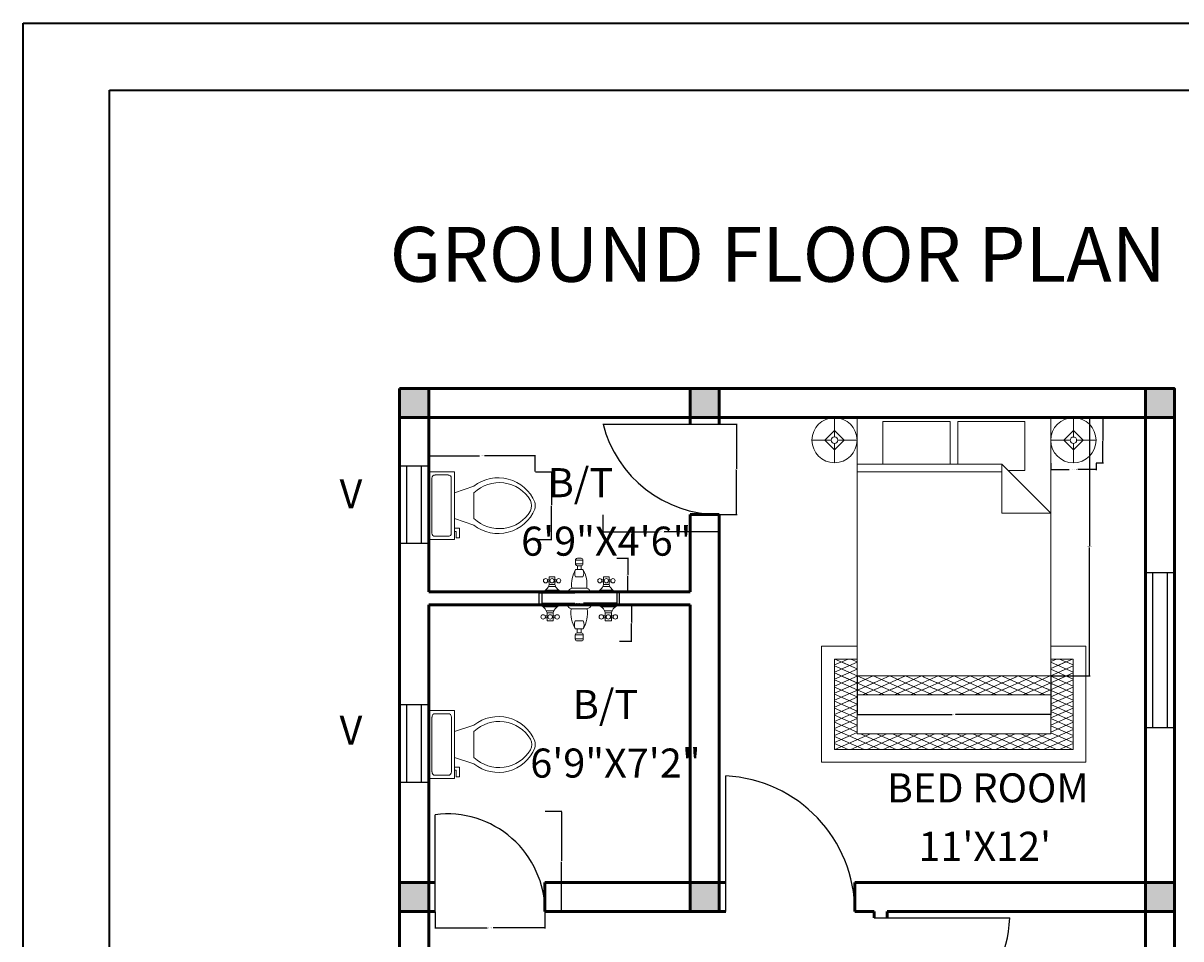
# Model space of a CAD drawing. Units: inches. Extents: x 28637 to 29820, y 17246 to 17928.
# Tile 2 of 6: x 28637 to 28996, y 17644 to 17928. Entities that reach past the tile are written whole.
import ezdxf

# ---------------------------------------------------------------- set-up
doc = ezdxf.new("R2010")
doc.units = ezdxf.units.IN
for name, color, linetype, lineweight in [('A-ANNO-DIMS', 2, 'Continuous', 18), ('A-ANNO-TEXT', 7, 'Continuous', 25), ('A-ANNO-TTLB', 7, 'Continuous', 35), ('A-AREA-IDEN', 30, 'Continuous', 25), ('A-COLS', 1, 'Continuous', 50), ('A-DOOR', 4, 'Continuous', 25), ('A-FLOR-FIXT', 8, 'Continuous', 18), ('A-FURN', 8, 'Continuous', 18), ('A-GLAZ', 4, 'Continuous', 25), ('A-WALL', 7, 'Continuous', 50)]:
    doc.layers.add(name, color=color, linetype=linetype, lineweight=lineweight)
doc.styles.get("Standard").update_dxf_attribs({"font": 'arial.ttf'})
doc.dimstyles.get("Standard").update_dxf_attribs({"dimtxt": 0.18, "dimasz": 0.18, "dimexe": 0.18, "dimexo": 0.0625, "dimgap": 0.09, "dimtad": 0, "dimtih": 1, "dimtoh": 1, "dimdec": 4, "dimzin": 0, "dimdsep": 46, "dimtxsty": 'Standard', "dimcen": 0.09, "dimadec": 0, "dimazin": 0, "dimtfac": 1, "dimtdec": 4, "dimtofl": 0, "dimtmove": 0, "dimatfit": 3, "dimfxl": 1, "dimtolj": 1, "dimtzin": 0, "dimarcsym": 0})

# ---------------------------------------------------------------- blocks, each defined once
blk = doc.blocks.new('Bed - Queen')
for p, q in [((0, -80.00003), (0, 0)), ((0, 0), (59.99999, 0)), ((59.99999, 0), (59.99999, -80.00003)), ((7.99999, -1.2), (28.79998, -1.2)), ((7.99999, -14.4), (7.99999, -1.2)), ((28.79998, -1.2), (28.79998, -14.4)), ((31.19999, -1.2), (51.99999, -1.2)), ((31.19999, -14.4), (31.19999, -1.2)), ((51.99999, -1.2), (51.99999, -16.4)), ((0, -14.4), (44.8, -14.4)), ((44.8, -16.8), (0, -16.8)), ((59.99999, -29.6), (44.8, -14.4)), ((44.8, -14.4), (44.8, -29.6)), ((51.99999, -16.4), (46.79936, -16.4)), ((44.8, -29.6), (59.99999, -29.6)), ((59.99999, -80.00003), (0, -80.00003))]:
    blk.add_line(p, q)
blk = doc.blocks.new('Lamp - Table')
for p, q in [((0, 7), (0, 1)), ((-1, 0), (-7, 0)), ((0, 3), (-3, 0)), ((-3, 0), (0, -3)), ((3, 0), (0, 3)), ((0, -3), (3, 0)), ((1, 0), (7, 0)), ((0, -1), (0, -7))]:
    blk.add_line(p, q)
for radius in [7, 1]:
    blk.add_circle((0, 0), radius)
blk = doc.blocks.new('Toilet - top')
for p, q in [((9.5, -6), (9.5, -2)), ((-10, -8.5), (-8, -8.5)), ((-10, -9.5), (-10, -8.5)), ((-7, -9.5), (-10, -9.5)), ((-8, -8.5), (-8, -8)), ((-7, -8), (-7, -9.5)), ((-4, -8), (-6, -14)), ((4, -8), (6, -14)), ((4, -14), (-4, -14))]:
    blk.add_line(p, q)
blk.add_lwpolyline([(10.5, -8), (10.5, 0), (-10.5, 0), (-10.5, -8)], close=True)
for points in [[(-9.5, -2), (-9.5, -6)], [(8.5, -1), (-8.5, -1)], [(-8.5, -7), (8.5, -7)]]:
    blk.add_lwpolyline(points)
for centre, radius, start, end in [((-8.62, -1.88), 0.884, 81.8699, 188.1301), ((8.62, -1.88), 0.884, 351.8699, 98.1301), ((-8.62, -6.12), 0.884, 171.8699, 278.1301), ((8.62, -6.12), 0.884, 261.8699, 8.1301), ((3.52, -21.58), 12.17, 141.4691, 247.9714), ((4.2, -21.82), 11.33, 136.3677, 238.9468), ((-3.52, -21.58), 12.17, 292.0284, 38.5307), ((-4.2, -21.82), 11.33, 301.053, 43.6321), ((0, -27.88), 4, 245.7318, 294.2682), ((0, -29), 4, 254.8605, 285.1395)]:
    blk.add_arc(centre, radius, start, end)
blk = doc.blocks.new('Faucet - Bathroom front')
for p, q in [((-0.5, 4.25), (0.5, 4.25)), ((0.5, 3.75), (-0.5, 3.75)), ((-0.5, 3), (0.5, 3)), ((-0.25, 3), (-0.25, 3.5)), ((0.25, 3.5), (0.25, 3)), ((-4, 1.625), (-4.25, 1.625)), ((-3.25, 1.625), (-3, 1.625)), ((0.5, 2), (-0.5, 2)), ((3.25, 1.625), (3, 1.625)), ((4, 1.625), (4.25, 1.625)), ((-5, 0), (-2.25, 0)), ((-4.5087, 0.25), (-2.7408, 0.25)), ((-4, 1.375), (-4.25, 1.375)), ((-3.1442, 0.75), (-4.0979, 0.75)), ((-3.25, 1.375), (-3, 1.375)), ((-1.5, 0), (1.5, 0)), ((-1, 0.5), (1, 0.5)), ((2.25, 0), (5, 0)), ((2.7413, 0.25), (4.5092, 0.25)), ((3.25, 1.375), (3, 1.375)), ((4.1058, 0.75), (3.1521, 0.75)), ((4, 1.375), (4.25, 1.375))]:
    blk.add_line(p, q)
for points in [[(-0.25, 4.5), (0.25, 4.5)], [(-0.5, 3.75), (-0.5, 4.25)], [(0.25, 3.5), (-0.25, 3.5)], [(0.5, 4.25), (0.5, 3.75)]]:
    blk.add_lwpolyline(points)
for points in [[(-4, 1), (-4, 2), (-3.25, 2), (-3.25, 1)], [(3.25, 1), (3.25, 2), (4, 2), (4, 1)]]:
    blk.add_lwpolyline(points, close=True)
for centre in [(-4.5, 1.5), (-3.625, 1.5), (-2.75, 1.5), (2.75, 1.5), (3.625, 1.5), (4.5, 1.5)]:
    blk.add_circle(centre, 0.2795)
for centre, radius, start, end in [((-0.2575, 4.2575), 0.2426, 88.22243, 181.7776), ((0.2575, 4.2575), 0.2426, 358.2224, 91.77757), ((3, 1), 4.0311, 150.2551, 187.125), ((0.6413, 2.5), 1.246, 156.3417, 203.6583), ((-0.2575, 3.7425), 0.2426, 178.2224, 271.7776), ((0.2575, 3.7425), 0.2426, 268.2224, 1.777565), ((-3, 1), 4.0311, 352.875, 29.74488), ((-0.6413, 2.5), 1.246, 336.3417, 23.65835), ((-5.375, 1.375), 1.4252, 285.2551, 344.7449), ((-1.875, 1.375), 1.4252, 195.2551, 254.7449), ((-0.7962, -0.2038), 0.7327, 106.1502, 163.8498), ((0.7962, -0.2038), 0.7327, 16.1502, 73.84979), ((1.875, 1.375), 1.4252, 285.2551, 344.7449), ((5.375, 1.375), 1.4252, 195.2551, 254.7449)]:
    blk.add_arc(centre, radius, start, end)
blk = doc.blocks.new('DOOR-42')
blk.add_line((28900.64, 17650.75), (28942.64, 17650.75))
blk.add_arc((28900.64, 17652.8), 42.05, 270, 357.2056)
blk = doc.blocks.new('DOOR-37')
blk.add_line((28816.64, 17803.75), (28852.64, 17803.75))
blk.add_arc((28852.64, 17812.9), 37.14, 194.25, 270)
blk = doc.blocks.new('DOOR-30')
blk.add_line((28764.64, 17652.75), (28764.64, 17682.75))
blk.add_arc((28768.41, 17652.75), 30.24, 0, 97.1527)
blk = doc.blocks.new('*D20')
at = {"layer": 'A-ANNO-DIMS', "color": 0, "lineweight": -2, "transparency": 16777216}
for p, q in [((28955.41, 17805.75), (28967.53, 17805.75)), ((28967.35, 17805.57), (28967.35, 17765.94)), ((28967.35, 17725.93), (28967.35, 17765.56)), ((28955.41, 17725.75), (28967.53, 17725.75))]:
    blk.add_line(p, q, dxfattribs=at)
at = {"layer": 'A-ANNO-DIMS', "color": 0, "transparency": 16777216}
for points in [[(28967.32, 17805.57), (28967.38, 17805.57), (28967.35, 17805.75)], [(28967.32, 17725.93), (28967.38, 17725.93), (28967.35, 17725.75)]]:
    blk.add_solid(points, dxfattribs=at)
at = {"layer": 'Defpoints', "color": 0, "transparency": 16777216}
for p in [(28955.35, 17805.75), (28967.35, 17805.75), (28955.35, 17725.75)]:
    blk.add_point(p, dxfattribs=at)
at = {"layer": 'A-ANNO-DIMS', "color": 0, "transparency": 16777216, "insert": (28967.35, 17765.75), "char_height": 0.18, "attachment_point": 5}
blk.add_mtext('\\A1;QUEEN BED 80 TYP.', dxfattribs=at)
blk = doc.blocks.new('*D21')
at = {"layer": 'A-ANNO-DIMS', "color": 0, "lineweight": -2, "transparency": 16777216}
for p, q in [((28895.35, 17725.69), (28895.35, 17713.57)), ((28955.35, 17725.69), (28955.35, 17713.57)), ((28895.53, 17713.75), (28924.82, 17713.75)), ((28955.17, 17713.75), (28925.88, 17713.75))]:
    blk.add_line(p, q, dxfattribs=at)
at = {"layer": 'A-ANNO-DIMS', "color": 0, "transparency": 16777216}
for points in [[(28895.53, 17713.78), (28895.53, 17713.72), (28895.35, 17713.75)], [(28955.17, 17713.78), (28955.17, 17713.72), (28955.35, 17713.75)]]:
    blk.add_solid(points, dxfattribs=at)
at = {"layer": 'Defpoints', "color": 0, "transparency": 16777216}
for p in [(28895.35, 17725.75), (28955.35, 17725.75), (28955.35, 17713.75)]:
    blk.add_point(p, dxfattribs=at)
at = {"layer": 'A-ANNO-DIMS', "color": 0, "transparency": 16777216, "insert": (28925.35, 17713.75), "char_height": 0.18, "attachment_point": 5}
blk.add_mtext('\\A1;60 TYP.', dxfattribs=at)
blk = doc.blocks.new('*D24')
at = {"layer": 'A-ANNO-DIMS', "color": 0, "lineweight": -2, "transparency": 16777216}
for p, q in [((28762.64, 17789.05), (28762.64, 17794.13)), ((28762.82, 17793.95), (28778.39, 17793.95)), ((28795.5, 17793.95), (28779.94, 17793.95)), ((28795.68, 17789.05), (28795.68, 17794.13))]:
    blk.add_line(p, q, dxfattribs=at)
at = {"layer": 'A-ANNO-DIMS', "color": 0, "transparency": 16777216}
for points in [[(28762.82, 17793.98), (28762.82, 17793.92), (28762.64, 17793.95)], [(28795.5, 17793.98), (28795.5, 17793.92), (28795.68, 17793.95)]]:
    blk.add_solid(points, dxfattribs=at)
at = {"layer": 'Defpoints', "color": 0, "transparency": 16777216}
for p in [(28762.64, 17793.95), (28762.64, 17788.99), (28795.68, 17788.99)]:
    blk.add_point(p, dxfattribs=at)
at = {"layer": 'A-ANNO-DIMS', "color": 0, "transparency": 16777216, "insert": (28779.16, 17793.95), "char_height": 0.18, "attachment_point": 5}
blk.add_mtext('\\A1;WC 33 TYP.', dxfattribs=at)
blk = doc.blocks.new('*D25')
at = {"layer": 'A-ANNO-DIMS', "color": 0, "lineweight": -2, "transparency": 16777216}
for p, q in [((28795.75, 17788.99), (28800.82, 17788.99)), ((28800.64, 17788.81), (28800.64, 17778.67)), ((28800.64, 17768.17), (28800.64, 17778.31)), ((28795.75, 17767.99), (28800.82, 17767.99))]:
    blk.add_line(p, q, dxfattribs=at)
at = {"layer": 'A-ANNO-DIMS', "color": 0, "transparency": 16777216}
for points in [[(28800.61, 17788.81), (28800.67, 17788.81), (28800.64, 17788.99)], [(28800.61, 17768.17), (28800.67, 17768.17), (28800.64, 17767.99)]]:
    blk.add_solid(points, dxfattribs=at)
at = {"layer": 'Defpoints', "color": 0, "transparency": 16777216}
for p in [(28795.68, 17788.99), (28800.64, 17788.99), (28795.68, 17767.99)]:
    blk.add_point(p, dxfattribs=at)
at = {"layer": 'A-ANNO-DIMS', "color": 0, "transparency": 16777216, "insert": (28800.64, 17778.49), "char_height": 0.18, "attachment_point": 5}
blk.add_mtext('\\A1;21 TYP.', dxfattribs=at)
blk = doc.blocks.new('*D26')
at = {"layer": 'A-ANNO-DIMS', "color": 0, "lineweight": -2, "transparency": 16777216}
for p, q in [((28955.35, 17791.69), (28955.35, 17789.47)), ((28969.35, 17791.69), (28969.35, 17789.47)), ((28955.53, 17789.65), (28961.01, 17789.65)), ((28969.17, 17789.65), (28963.69, 17789.65))]:
    blk.add_line(p, q, dxfattribs=at)
at = {"layer": 'A-ANNO-DIMS', "color": 0, "transparency": 16777216}
for points in [[(28955.53, 17789.68), (28955.53, 17789.62), (28955.35, 17789.65)], [(28969.17, 17789.68), (28969.17, 17789.62), (28969.35, 17789.65)]]:
    blk.add_solid(points, dxfattribs=at)
at = {"layer": 'Defpoints', "color": 0, "transparency": 16777216}
for p in [(28955.35, 17791.75), (28969.35, 17791.75), (28969.35, 17789.65)]:
    blk.add_point(p, dxfattribs=at)
at = {"layer": 'A-ANNO-DIMS', "color": 0, "transparency": 16777216, "insert": (28962.35, 17789.65), "char_height": 0.18, "attachment_point": 5}
blk.add_mtext('\\A1;TABLE LAMP 14 TYP.', dxfattribs=at)
blk = doc.blocks.new('*D27')
at = {"layer": 'A-ANNO-DIMS', "color": 0, "lineweight": -2, "transparency": 16777216}
for p, q in [((28969.41, 17805.75), (28971.63, 17805.75)), ((28971.45, 17805.57), (28971.45, 17798.93)), ((28971.45, 17791.93), (28971.45, 17798.57)), ((28969.41, 17791.75), (28971.63, 17791.75))]:
    blk.add_line(p, q, dxfattribs=at)
at = {"layer": 'A-ANNO-DIMS', "color": 0, "transparency": 16777216}
for points in [[(28971.42, 17805.57), (28971.48, 17805.57), (28971.45, 17805.75)], [(28971.42, 17791.93), (28971.48, 17791.93), (28971.45, 17791.75)]]:
    blk.add_solid(points, dxfattribs=at)
at = {"layer": 'Defpoints', "color": 0, "transparency": 16777216}
for p in [(28969.35, 17805.75), (28971.45, 17805.75), (28969.35, 17791.75)]:
    blk.add_point(p, dxfattribs=at)
at = {"layer": 'A-ANNO-DIMS', "color": 0, "transparency": 16777216, "insert": (28971.45, 17798.75), "char_height": 0.18, "attachment_point": 5}
blk.add_mtext('\\A1;14 TYP.', dxfattribs=at)
blk = doc.blocks.new('*D30')
at = {"layer": 'A-ANNO-DIMS', "color": 0, "lineweight": -2, "transparency": 16777216}
for p, q in [((28797.68, 17751.69), (28797.68, 17748.09)), ((28820.88, 17751.69), (28820.88, 17748.09)), ((28797.86, 17748.27), (28807.93, 17748.27)), ((28820.7, 17748.27), (28810.64, 17748.27))]:
    blk.add_line(p, q, dxfattribs=at)
at = {"layer": 'A-ANNO-DIMS', "color": 0, "transparency": 16777216}
for points in [[(28797.86, 17748.3), (28797.86, 17748.24), (28797.68, 17748.27)], [(28820.7, 17748.3), (28820.7, 17748.24), (28820.88, 17748.27)]]:
    blk.add_solid(points, dxfattribs=at)
at = {"layer": 'Defpoints', "color": 0, "transparency": 16777216}
for p in [(28797.68, 17751.75), (28820.88, 17751.75), (28820.88, 17748.27)]:
    blk.add_point(p, dxfattribs=at)
at = {"layer": 'A-ANNO-DIMS', "color": 0, "transparency": 16777216, "insert": (28809.28, 17748.27), "char_height": 0.18, "attachment_point": 5}
blk.add_mtext('\\A1;WASH BASIN 23 TYP.', dxfattribs=at)
blk = doc.blocks.new('*D31')
at = {"layer": 'A-ANNO-DIMS', "color": 0, "lineweight": -2, "transparency": 16777216}
for p, q in [((28820.94, 17762.2), (28824.54, 17762.2)), ((28824.36, 17762.02), (28824.36, 17757.16)), ((28824.36, 17751.93), (28824.36, 17756.79)), ((28820.94, 17751.75), (28824.54, 17751.75))]:
    blk.add_line(p, q, dxfattribs=at)
at = {"layer": 'A-ANNO-DIMS', "color": 0, "transparency": 16777216}
for points in [[(28824.33, 17762.02), (28824.39, 17762.02), (28824.36, 17762.2)], [(28824.33, 17751.93), (28824.39, 17751.93), (28824.36, 17751.75)]]:
    blk.add_solid(points, dxfattribs=at)
at = {"layer": 'Defpoints', "color": 0, "transparency": 16777216}
for p in [(28820.88, 17762.2), (28824.36, 17762.2), (28820.88, 17751.75)]:
    blk.add_point(p, dxfattribs=at)
at = {"layer": 'A-ANNO-DIMS', "color": 0, "transparency": 16777216, "insert": (28824.36, 17756.97), "char_height": 0.18, "attachment_point": 5}
blk.add_mtext('\\A1;10 TYP.', dxfattribs=at)
blk = doc.blocks.new('*D32')
at = {"layer": 'A-ANNO-DIMS', "color": 0, "lineweight": -2, "transparency": 16777216}
for p, q in [((28796.85, 17747.81), (28796.85, 17751.66)), ((28797.03, 17751.48), (28807.93, 17751.48)), ((28821.53, 17751.48), (28810.64, 17751.48)), ((28821.71, 17747.81), (28821.71, 17751.66))]:
    blk.add_line(p, q, dxfattribs=at)
at = {"layer": 'A-ANNO-DIMS', "color": 0, "transparency": 16777216}
for points in [[(28797.03, 17751.51), (28797.03, 17751.45), (28796.85, 17751.48)], [(28821.53, 17751.51), (28821.53, 17751.45), (28821.71, 17751.48)]]:
    blk.add_solid(points, dxfattribs=at)
at = {"layer": 'Defpoints', "color": 0, "transparency": 16777216}
for p in [(28821.71, 17751.48), (28796.85, 17747.75), (28821.71, 17747.75)]:
    blk.add_point(p, dxfattribs=at)
at = {"layer": 'A-ANNO-DIMS', "color": 0, "transparency": 16777216, "insert": (28809.28, 17751.48), "char_height": 0.18, "attachment_point": 5}
blk.add_mtext('\\A1;WASH BASIN 25 TYP.', dxfattribs=at)
blk = doc.blocks.new('*D33')
at = {"layer": 'A-ANNO-DIMS', "color": 0, "lineweight": -2, "transparency": 16777216}
for p, q in [((28821.77, 17747.75), (28825.62, 17747.75)), ((28825.44, 17747.57), (28825.44, 17742.33)), ((28825.44, 17736.74), (28825.44, 17741.97)), ((28821.77, 17736.56), (28825.62, 17736.56))]:
    blk.add_line(p, q, dxfattribs=at)
at = {"layer": 'A-ANNO-DIMS', "color": 0, "transparency": 16777216}
for points in [[(28825.41, 17747.57), (28825.47, 17747.57), (28825.44, 17747.75)], [(28825.41, 17736.74), (28825.47, 17736.74), (28825.44, 17736.56)]]:
    blk.add_solid(points, dxfattribs=at)
at = {"layer": 'Defpoints', "color": 0, "transparency": 16777216}
for p in [(28821.71, 17747.75), (28821.71, 17736.56), (28825.44, 17736.56)]:
    blk.add_point(p, dxfattribs=at)
at = {"layer": 'A-ANNO-DIMS', "color": 0, "transparency": 16777216, "insert": (28825.44, 17742.15), "char_height": 0.18, "attachment_point": 5}
blk.add_mtext('\\A1;11 TYP.', dxfattribs=at)
blk = doc.blocks.new('*D38')
at = {"layer": 'A-ANNO-DIMS', "color": 0, "lineweight": -2, "transparency": 16777216}
for p, q in [((28816.64, 17775.69), (28816.64, 17770.17)), ((28852.64, 17775.69), (28852.64, 17770.17)), ((28816.82, 17770.35), (28833.71, 17770.35)), ((28852.46, 17770.35), (28835.58, 17770.35))]:
    blk.add_line(p, q, dxfattribs=at)
at = {"layer": 'A-ANNO-DIMS', "color": 0, "transparency": 16777216}
for points in [[(28816.82, 17770.38), (28816.82, 17770.32), (28816.64, 17770.35)], [(28852.46, 17770.38), (28852.46, 17770.32), (28852.64, 17770.35)]]:
    blk.add_solid(points, dxfattribs=at)
at = {"layer": 'Defpoints', "color": 0, "transparency": 16777216}
for p in [(28816.64, 17775.75), (28852.64, 17775.75), (28852.64, 17770.35)]:
    blk.add_point(p, dxfattribs=at)
at = {"layer": 'A-ANNO-DIMS', "color": 0, "transparency": 16777216, "insert": (28834.64, 17770.35), "char_height": 0.18, "attachment_point": 5}
blk.add_mtext('\\A1;DOOR 36 TYP.', dxfattribs=at)
blk = doc.blocks.new('*D39')
at = {"layer": 'A-ANNO-DIMS', "color": 0, "lineweight": -2, "transparency": 16777216}
for p, q in [((28852.71, 17803.75), (28858.22, 17803.75)), ((28858.04, 17803.57), (28858.04, 17789.93)), ((28858.04, 17775.93), (28858.04, 17789.57)), ((28852.71, 17775.75), (28858.22, 17775.75))]:
    blk.add_line(p, q, dxfattribs=at)
at = {"layer": 'A-ANNO-DIMS', "color": 0, "transparency": 16777216}
for points in [[(28858.01, 17803.57), (28858.07, 17803.57), (28858.04, 17803.75)], [(28858.01, 17775.93), (28858.07, 17775.93), (28858.04, 17775.75)]]:
    blk.add_solid(points, dxfattribs=at)
at = {"layer": 'Defpoints', "color": 0, "transparency": 16777216}
for p in [(28852.64, 17803.75), (28858.04, 17803.75), (28852.64, 17775.75)]:
    blk.add_point(p, dxfattribs=at)
at = {"layer": 'A-ANNO-DIMS', "color": 0, "transparency": 16777216, "insert": (28858.04, 17789.75), "char_height": 0.18, "attachment_point": 5}
blk.add_mtext('\\A1;28 TYP.', dxfattribs=at)
blk = doc.blocks.new('*D40')
at = {"layer": 'A-ANNO-DIMS', "color": 0, "lineweight": -2, "transparency": 16777216}
for p, q in [((28764.64, 17652.69), (28764.64, 17647.47)), ((28798.64, 17652.69), (28798.64, 17647.47)), ((28764.82, 17647.65), (28780.71, 17647.65)), ((28798.46, 17647.65), (28782.58, 17647.65))]:
    blk.add_line(p, q, dxfattribs=at)
at = {"layer": 'A-ANNO-DIMS', "color": 0, "transparency": 16777216}
for points in [[(28764.82, 17647.68), (28764.82, 17647.62), (28764.64, 17647.65)], [(28798.46, 17647.68), (28798.46, 17647.62), (28798.64, 17647.65)]]:
    blk.add_solid(points, dxfattribs=at)
at = {"layer": 'Defpoints', "color": 0, "transparency": 16777216}
for p in [(28764.64, 17652.75), (28798.64, 17652.75), (28798.64, 17647.65)]:
    blk.add_point(p, dxfattribs=at)
at = {"layer": 'A-ANNO-DIMS', "color": 0, "transparency": 16777216, "insert": (28781.64, 17647.65), "char_height": 0.18, "attachment_point": 5}
blk.add_mtext('\\A1;DOOR 34 TYP.', dxfattribs=at)
blk = doc.blocks.new('*D41')
at = {"layer": 'A-ANNO-DIMS', "color": 0, "lineweight": -2, "transparency": 16777216}
for p, q in [((28798.71, 17683.83), (28803.92, 17683.83)), ((28803.74, 17683.65), (28803.74, 17668.47)), ((28803.74, 17652.93), (28803.74, 17668.11)), ((28798.71, 17652.75), (28803.92, 17652.75))]:
    blk.add_line(p, q, dxfattribs=at)
at = {"layer": 'A-ANNO-DIMS', "color": 0, "transparency": 16777216}
for points in [[(28803.71, 17683.65), (28803.77, 17683.65), (28803.74, 17683.83)], [(28803.71, 17652.93), (28803.77, 17652.93), (28803.74, 17652.75)]]:
    blk.add_solid(points, dxfattribs=at)
at = {"layer": 'Defpoints', "color": 0, "transparency": 16777216}
for p in [(28798.64, 17683.83), (28803.74, 17683.83), (28798.64, 17652.75)]:
    blk.add_point(p, dxfattribs=at)
at = {"layer": 'A-ANNO-DIMS', "color": 0, "transparency": 16777216, "insert": (28803.74, 17668.29), "char_height": 0.18, "attachment_point": 5}
blk.add_mtext('\\A1;31 TYP.', dxfattribs=at)

msp = doc.modelspace()

# ---------------------------------------------------------------- hatches: boundary and pattern name
at = {"layer": 'A-COLS'}
h = msp.add_hatch(color=256, dxfattribs=at)
h.dxf.hatch_style = 1
h.paths.add_polyline_path([(28753.64, 17814.75), (28753.64, 17805.75), (28762.64, 17805.75), (28762.64, 17814.75)])
h = msp.add_hatch(color=256, dxfattribs=at)
h.dxf.hatch_style = 1
h.paths.add_polyline_path([(28843.64, 17814.75), (28843.64, 17805.75), (28852.64, 17805.75), (28852.64, 17814.75)])
h = msp.add_hatch(color=256, dxfattribs=at)
h.dxf.hatch_style = 1
h.paths.add_polyline_path([(28993.64, 17814.75), (28984.64, 17814.75), (28984.64, 17805.75), (28993.64, 17805.75)])
h = msp.add_hatch(color=256, dxfattribs=at)
h.dxf.hatch_style = 1
h.paths.add_polyline_path([(28753.64, 17661.75), (28753.64, 17652.75), (28762.64, 17652.75), (28762.64, 17661.75)])
h = msp.add_hatch(color=256, dxfattribs=at)
h.dxf.hatch_style = 1
h.paths.add_polyline_path([(28843.64, 17661.75), (28843.64, 17652.75), (28852.64, 17652.75), (28852.64, 17661.75)])
h = msp.add_hatch(color=256, dxfattribs=at)
h.dxf.hatch_style = 1
h.paths.add_polyline_path([(28984.64, 17661.75), (28984.64, 17652.75), (28993.64, 17652.75), (28993.64, 17661.75)])

# ---------------------------------------------------------------- linework, layer by layer
at = {"layer": 'A-ANNO-TTLB'}
for points in [[(28637.03, 17927.97), (29820.02, 17927.97), (29820.02, 17246.37), (28637.03, 17246.37)], [(28663.78, 17907.18), (29794.75, 17907.18), (29794.75, 17268.65), (28663.78, 17268.65)]]:
    msp.add_lwpolyline(points, close=True, dxfattribs=at)
at = {"layer": 'A-COLS'}
for points in [[(28753.64, 17814.75), (28762.64, 17814.75), (28762.64, 17805.75), (28753.64, 17805.75)], [(28843.64, 17814.75), (28852.64, 17814.75), (28852.64, 17805.75), (28843.64, 17805.75)], [(28984.64, 17814.75), (28993.64, 17814.75), (28993.64, 17805.75), (28984.64, 17805.75)], [(28753.64, 17661.75), (28762.64, 17661.75), (28762.64, 17652.75), (28753.64, 17652.75)], [(28843.64, 17661.75), (28852.64, 17661.75), (28852.64, 17652.75), (28843.64, 17652.75)], [(28984.64, 17661.75), (28993.64, 17661.75), (28993.64, 17652.75), (28984.64, 17652.75)]]:
    msp.add_lwpolyline(points, close=True, dxfattribs=at)
at = {"layer": 'A-FURN'}
for p, q in [((28884.35, 17734.98), (28895.35, 17734.98)), ((28884.35, 17734.98), (28884.35, 17698.98)), ((28955.35, 17734.98), (28966.24, 17734.98)), ((28966.24, 17734.98), (28966.24, 17698.98)), ((28888.35, 17730.98), (28888.35, 17702.98)), ((28888.35, 17730.98), (28895.35, 17730.98)), ((28888.35, 17729.14), (28892.54, 17730.98)), ((28888.35, 17726.95), (28895.35, 17730.03)), ((28888.48, 17730.98), (28895.35, 17727.96)), ((28890.76, 17729.97), (28895.35, 17727.96)), ((28893.45, 17730.98), (28895.35, 17730.14)), ((28893.45, 17730.98), (28895.35, 17730.14)), ((28955.35, 17730.98), (28962.24, 17730.98)), ((28955.35, 17728), (28962.11, 17730.98)), ((28955.35, 17728), (28962.11, 17730.98)), ((28955.35, 17728), (28962.11, 17730.98)), ((28955.35, 17730.19), (28957.14, 17730.98)), ((28955.35, 17729.98), (28962.24, 17726.95)), ((28955.35, 17728), (28959.83, 17729.97)), ((28958.06, 17730.98), (28962.24, 17729.14)), ((28962.24, 17730.98), (28962.24, 17702.98)), ((28888.35, 17728.85), (28895.35, 17725.77)), ((28888.35, 17724.77), (28895.35, 17727.84)), ((28888.35, 17726.66), (28895.35, 17723.59)), ((28888.35, 17722.58), (28895.35, 17725.66)), ((28889.15, 17726.31), (28899.7, 17721.68)), ((28889.96, 17728.14), (28895.35, 17725.77)), ((28894.62, 17725.34), (28895.56, 17725.75)), ((28895.39, 17725.75), (28900.5, 17723.51)), ((28895.42, 17723.51), (28900.36, 17725.75)), ((28896.23, 17721.68), (28905.5, 17725.75)), ((28900.36, 17725.75), (28910.39, 17721.35)), ((28900.36, 17725.75), (28901.31, 17725.34)), ((28901.19, 17721.68), (28910.3, 17725.75)), ((28904.56, 17725.34), (28905.5, 17725.75)), ((28905.5, 17725.75), (28912.87, 17722.44)), ((28906.16, 17721.68), (28915.27, 17725.75)), ((28910.3, 17725.75), (28915.41, 17723.51)), ((28911.13, 17721.68), (28920.41, 17725.75)), ((28915.27, 17725.75), (28916.22, 17725.34)), ((28916.1, 17721.68), (28925.38, 17725.75)), ((28920.41, 17725.75), (28927.78, 17722.44)), ((28921.07, 17721.68), (28930.35, 17725.75)), ((28925.38, 17725.75), (28930.32, 17723.51)), ((28926.04, 17721.68), (28935.32, 17725.75)), ((28930.35, 17725.75), (28937.72, 17722.44)), ((28931.01, 17721.68), (28940.12, 17725.75)), ((28935.32, 17725.75), (28940.26, 17723.51)), ((28940.12, 17725.75), (28945.23, 17723.51)), ((28944.31, 17725.34), (28945.26, 17725.75)), ((28945.12, 17723.51), (28950.15, 17725.75)), ((28945.26, 17725.75), (28950.2, 17723.51)), ((28950.09, 17723.51), (28955.2, 17725.75)), ((28950.09, 17723.51), (28955.2, 17725.75)), ((28950.15, 17725.75), (28962.24, 17720.4)), ((28950.15, 17725.75), (28951.01, 17725.37)), ((28950.89, 17721.68), (28961.44, 17726.31)), ((28955.2, 17725.75), (28962.24, 17722.58)), ((28955.35, 17725.82), (28962.24, 17728.85)), ((28955.35, 17725.82), (28962.24, 17728.85)), ((28955.35, 17725.82), (28960.63, 17728.14)), ((28955.35, 17725.82), (28960.63, 17728.14)), ((28955.35, 17727.8), (28962.24, 17724.77)), ((28955.35, 17723.63), (28962.24, 17726.66)), ((28888.35, 17724.48), (28898.89, 17719.84)), ((28888.35, 17720.4), (28895.35, 17723.48)), ((28888.35, 17722.3), (28895.35, 17719.22)), ((28896.23, 17721.68), (28900.77, 17723.68)), ((28896.23, 17721.68), (28900.77, 17723.68)), ((28900.45, 17723.53), (28908.83, 17719.84)), ((28910.06, 17723.68), (28914.61, 17721.68)), ((28915.03, 17723.68), (28919.58, 17721.68)), ((28915.83, 17725.51), (28920.38, 17723.51)), ((28920, 17723.68), (28924.55, 17721.68)), ((28924.97, 17723.68), (28929.52, 17721.68)), ((28929.94, 17723.68), (28934.49, 17721.68)), ((28934.91, 17723.68), (28939.46, 17721.68)), ((28935.98, 17721.68), (28940.53, 17723.68)), ((28939.88, 17723.68), (28944.43, 17721.68)), ((28940.15, 17723.51), (28944.7, 17725.51)), ((28940.95, 17721.68), (28945.5, 17723.68)), ((28944.85, 17723.68), (28949.4, 17721.68)), ((28945.92, 17721.68), (28950.47, 17723.68)), ((28945.92, 17721.68), (28950.47, 17723.68)), ((28949.82, 17723.68), (28954.37, 17721.68)), ((28949.82, 17723.68), (28954.37, 17721.68)), ((28951.7, 17719.84), (28962.24, 17724.48)), ((28954.79, 17723.68), (28962.24, 17720.4)), ((28955.35, 17719.26), (28962.24, 17722.3)), ((28888.35, 17718.21), (28896.61, 17721.84)), ((28888.35, 17720.11), (28895.35, 17717.03)), ((28888.35, 17716.03), (28895.35, 17719.11)), ((28895.35, 17719.84), (28955.35, 17719.84)), ((28895.35, 17719.84), (28895.35, 17707.84)), ((28897.03, 17719.84), (28901.58, 17721.84)), ((28899.31, 17721.84), (28903.86, 17719.84)), ((28902, 17719.84), (28906.55, 17721.84)), ((28906.97, 17719.84), (28911.52, 17721.84)), ((28909.25, 17721.84), (28913.8, 17719.84)), ((28911.94, 17719.84), (28916.49, 17721.84)), ((28911.94, 17719.84), (28916.49, 17721.84)), ((28911.94, 17719.84), (28916.49, 17721.84)), ((28914.22, 17721.84), (28918.77, 17719.84)), ((28914.22, 17721.84), (28918.77, 17719.84)), ((28916.91, 17719.84), (28921.46, 17721.84)), ((28919.19, 17721.84), (28923.74, 17719.84)), ((28921.88, 17719.84), (28926.43, 17721.84)), ((28924.16, 17721.84), (28928.71, 17719.84)), ((28926.85, 17719.84), (28931.4, 17721.84)), ((28929.13, 17721.84), (28933.68, 17719.84)), ((28931.82, 17719.84), (28936.37, 17721.84)), ((28934.1, 17721.84), (28938.65, 17719.84)), ((28936.79, 17719.84), (28941.34, 17721.84)), ((28936.79, 17719.84), (28941.34, 17721.84)), ((28936.79, 17719.84), (28941.34, 17721.84)), ((28939.07, 17721.84), (28943.62, 17719.84)), ((28941.76, 17719.84), (28946.31, 17721.84)), ((28941.76, 17719.84), (28946.31, 17721.84)), ((28944.04, 17721.84), (28948.59, 17719.84)), ((28946.73, 17719.84), (28951.28, 17721.84)), ((28949.01, 17721.84), (28953.56, 17719.84)), ((28953.98, 17721.84), (28962.24, 17718.21)), ((28955.35, 17717.08), (28962.24, 17720.11)), ((28955.35, 17719.84), (28955.35, 17707.84)), ((28955.35, 17719.06), (28962.24, 17716.03)), ((28888.35, 17717.93), (28895.35, 17714.85)), ((28888.35, 17713.84), (28895.35, 17716.92)), ((28888.35, 17715.74), (28895.35, 17712.66)), ((28955.35, 17714.9), (28962.24, 17717.93)), ((28955.35, 17716.87), (28962.24, 17713.84)), ((28955.35, 17712.71), (28962.24, 17715.74)), ((28888.35, 17711.66), (28895.35, 17714.74)), ((28888.35, 17713.56), (28895.35, 17710.48)), ((28888.35, 17709.47), (28895.35, 17712.55)), ((28888.35, 17711.37), (28895.35, 17708.29)), ((28955.35, 17714.69), (28962.24, 17711.66)), ((28955.35, 17710.53), (28962.24, 17713.56)), ((28955.35, 17712.51), (28962.24, 17709.47)), ((28955.35, 17708.34), (28962.24, 17711.37)), ((28888.35, 17707.29), (28895.35, 17710.37)), ((28888.35, 17709.19), (28902.48, 17702.98)), ((28888.35, 17705.11), (28895.35, 17708.18)), ((28888.48, 17702.98), (28899.55, 17707.84)), ((28893.45, 17702.98), (28904.52, 17707.84)), ((28895.35, 17707.84), (28955.35, 17707.84)), ((28896.37, 17707.84), (28907.44, 17702.98)), ((28898.42, 17702.98), (28909.49, 17707.84)), ((28898.42, 17702.98), (28909.49, 17707.84)), ((28898.42, 17702.98), (28909.49, 17707.84)), ((28901.34, 17707.84), (28912.41, 17702.98)), ((28903.39, 17702.98), (28914.46, 17707.84)), ((28903.39, 17702.98), (28914.46, 17707.84)), ((28906.31, 17707.84), (28917.38, 17702.98)), ((28908.36, 17702.98), (28919.43, 17707.84)), ((28911.28, 17707.84), (28922.35, 17702.98)), ((28913.33, 17702.98), (28924.4, 17707.84)), ((28916.25, 17707.84), (28927.32, 17702.98)), ((28918.3, 17702.98), (28929.37, 17707.84)), ((28921.22, 17707.84), (28932.29, 17702.98)), ((28923.27, 17702.98), (28934.34, 17707.84)), ((28926.19, 17707.84), (28937.26, 17702.98)), ((28928.24, 17702.98), (28939.31, 17707.84)), ((28931.16, 17707.84), (28942.23, 17702.98)), ((28933.21, 17702.98), (28944.28, 17707.84)), ((28936.13, 17707.84), (28947.2, 17702.98)), ((28938.18, 17702.98), (28949.25, 17707.84)), ((28941.1, 17707.84), (28952.17, 17702.98)), ((28943.15, 17702.98), (28954.22, 17707.84)), ((28946.07, 17707.84), (28957.14, 17702.98)), ((28946.07, 17707.84), (28957.14, 17702.98)), ((28948.12, 17702.98), (28962.24, 17709.19)), ((28951.04, 17707.84), (28962.11, 17702.98)), ((28955.35, 17710.32), (28962.24, 17707.29)), ((28955.35, 17708.14), (28962.24, 17705.11)), ((28888.35, 17707), (28897.51, 17702.98)), ((28888.35, 17704.82), (28892.54, 17702.98)), ((28953.09, 17702.98), (28962.24, 17707)), ((28958.06, 17702.98), (28962.24, 17704.82)), ((28888.35, 17702.98), (28962.24, 17702.98)), ((28884.35, 17698.98), (28966.24, 17698.98))]:
    msp.add_line(p, q, dxfattribs=at)
at = {"layer": 'A-GLAZ'}
for p, q in [((28762.64, 17790.75), (28753.64, 17790.75)), ((28755.89, 17766.75), (28755.89, 17790.75)), ((28760.39, 17766.75), (28760.39, 17790.75)), ((28762.64, 17766.75), (28753.64, 17766.75)), ((28984.64, 17757.75), (28993.64, 17757.75)), ((28986.89, 17757.75), (28986.89, 17709.75)), ((28991.39, 17757.75), (28991.39, 17709.75)), ((28762.64, 17716.75), (28753.64, 17716.75)), ((28755.89, 17692.75), (28755.89, 17716.75)), ((28760.39, 17692.75), (28760.39, 17716.75)), ((28984.64, 17709.75), (28993.64, 17709.75)), ((28762.64, 17692.75), (28753.64, 17692.75))]:
    msp.add_line(p, q, dxfattribs=at)
at = {"layer": 'A-WALL'}
for p, q in [((28753.64, 17814.75), (28993.64, 17814.75)), ((28753.64, 17334.75), (28753.64, 17814.75)), ((28993.64, 17814.75), (28993.64, 17334.75)), ((28762.64, 17805.75), (28843.64, 17805.75)), ((28762.64, 17751.75), (28762.64, 17805.75)), ((28843.64, 17805.75), (28843.64, 17803.75)), ((28843.64, 17805.75), (28843.64, 17803.75)), ((28852.64, 17805.75), (28852.64, 17803.75)), ((28852.64, 17805.75), (28852.64, 17803.75)), ((28852.64, 17805.75), (28984.64, 17805.75)), ((28984.64, 17805.75), (28984.64, 17661.75)), ((28843.64, 17775.75), (28852.64, 17775.75)), ((28843.64, 17775.75), (28843.64, 17751.75)), ((28843.64, 17775.75), (28843.64, 17751.75)), ((28852.64, 17775.75), (28852.64, 17661.75)), ((28852.64, 17775.75), (28852.64, 17661.75)), ((28762.64, 17751.75), (28843.64, 17751.75)), ((28762.64, 17747.75), (28843.64, 17747.75)), ((28762.64, 17661.75), (28762.64, 17747.75)), ((28843.64, 17747.75), (28843.64, 17661.75)), ((28843.64, 17747.75), (28843.64, 17661.75)), ((28762.64, 17661.75), (28764.64, 17661.75)), ((28798.64, 17652.75), (28798.64, 17661.75)), ((28798.64, 17661.75), (28843.64, 17661.75)), ((28852.64, 17661.75), (28854.64, 17661.75)), ((28894.64, 17661.75), (28894.64, 17652.75)), ((28894.64, 17661.75), (28984.64, 17661.75)), ((28762.64, 17652.75), (28764.64, 17652.75)), ((28762.64, 17508.75), (28762.64, 17652.75)), ((28798.64, 17652.75), (28854.64, 17652.75)), ((28894.64, 17652.75), (28900.64, 17652.75)), ((28900.64, 17652.75), (28900.64, 17650.75)), ((28904.64, 17652.75), (28904.64, 17650.75)), ((28904.64, 17652.75), (28984.64, 17652.75)), ((28984.64, 17652.75), (28984.64, 17508.75))]:
    msp.add_line(p, q, dxfattribs=at)

# ---------------------------------------------------------------- block references
at = {"layer": 'A-DOOR'}
for name in ['DOOR-37', 'DOOR-30', 'DOOR-42']:
    msp.add_blockref(name, (0, 0), dxfattribs=at)
at = {"layer": 'A-DOOR', "rotation": 89.99999999999737}
msp.add_blockref('DOOR-42', (46505.4, -11247.89), dxfattribs=at)
at = {"layer": 'A-FLOR-FIXT', "rotation": 90}
for p in [(28762.64, 17778.49), (28762.67, 17704.5)]:
    msp.add_blockref('Toilet - top', p, dxfattribs=at)
at = {"layer": 'A-FLOR-FIXT', "xscale": 2.319878252974637, "yscale": 2.319878252974637, "zscale": 2.319878252974637}
msp.add_blockref('Faucet - Bathroom front', (28809.28, 17751.75), dxfattribs=at)
at = {"layer": 'A-FLOR-FIXT', "xscale": -2.485809345179645, "yscale": 2.485809345179645, "zscale": 2.485809345179645, "rotation": 180}
msp.add_blockref('Faucet - Bathroom front', (28809.28, 17747.75), dxfattribs=at)
at = {"layer": 'A-FURN'}
for name, p in [('Lamp - Table', (28888.35, 17798.77)), ('Bed - Queen', (28895.35, 17805.75)), ('Lamp - Table', (28962.35, 17798.75))]:
    msp.add_blockref(name, p, dxfattribs=at)

# ---------------------------------------------------------------- texts
at = {"layer": 'A-ANNO-TEXT'}
for s, height, p in [('GROUND FLOOR PLAN', 17, (28750.56, 17847.85)), ('    V', 9, (28724.03, 17777.69)), ('    V', 9, (28724.03, 17704.44))]:
    msp.add_text(s, height=height, dxfattribs=at).set_placement(p)
at = {"layer": 'A-AREA-IDEN'}
for s, p in [('    B/T', (28788.53, 17781.11)), (' 6\'9"X4\'6"', (28788.53, 17762.99)), ('   B/T', (28799.04, 17712.42)), ('6\'9"X7\'2"', (28794.11, 17694.24)), ('BED ROOM', (28904.58, 17686.56)), (" 11'X12'", (28911.58, 17668.45))]:
    msp.add_text(s, height=9, dxfattribs=at).set_placement(p)

# ---------------------------------------------------------------- dimensions: what is measured, and where the dimension line sits
at = {"layer": 'A-ANNO-DIMS'}
for base, p1, p2, angle, text, picture, middle in [((28967.35, 17805.75), (28955.35, 17725.75), (28955.35, 17805.75), 90, 'QUEEN BED <> TYP.', '*D20', (28967.35, 17765.75)), ((28971.45, 17805.75), (28969.35, 17791.75), (28969.35, 17805.75), 90, '<> TYP.', '*D27', (28971.45, 17798.75)), ((28858.04, 17803.75), (28852.64, 17775.75), (28852.64, 17803.75), 90, '<> TYP.', '*D39', (28858.04, 17789.75)), ((28762.64, 17793.95), (28795.68, 17788.99), (28762.64, 17788.99), 180, 'WC <> TYP.', '*D24', (28779.16, 17793.95)), ((28800.64, 17788.99), (28795.68, 17767.99), (28795.68, 17788.99), 90, '<> TYP.', '*D25', (28800.64, 17778.49)), ((28824.36, 17762.2), (28820.88, 17751.75), (28820.88, 17762.2), 90, '<> TYP.', '*D31', (28824.36, 17756.97)), ((28825.44, 17736.56), (28821.71, 17747.75), (28821.71, 17736.56), 270, '<> TYP.', '*D33', (28825.44, 17742.15)), ((28803.74, 17683.83), (28798.64, 17652.75), (28798.64, 17683.83), 90, '<> TYP.', '*D41', (28803.74, 17668.29))]:
    dim = msp.add_linear_dim(base=base, p1=p1, p2=p2, angle=angle, text=text, dimstyle='Standard', override={"dimdec": 0, "dimlfac": 1, "dimrnd": 0, "dimzin": 0, "dimdsep": 46, "dimlunit": 2}, dxfattribs=at)
    dim.commit()
    dim.dimension.update_dxf_attribs({"geometry": picture, "text_midpoint": middle})
for base, p1, p2, text, picture, middle in [((28969.35, 17789.65), (28955.35, 17791.75), (28969.35, 17791.75), 'TABLE LAMP <> TYP.', '*D26', (28962.35, 17789.65)), ((28852.64, 17770.35), (28816.64, 17775.75), (28852.64, 17775.75), 'DOOR <> TYP.', '*D38', (28834.64, 17770.35)), ((28821.71, 17751.48), (28796.85, 17747.75), (28821.71, 17747.75), 'WASH BASIN <> TYP.', '*D32', (28809.28, 17751.48)), ((28820.88, 17748.27), (28797.68, 17751.75), (28820.88, 17751.75), 'WASH BASIN <> TYP.', '*D30', (28809.28, 17748.27)), ((28955.35, 17713.75), (28895.35, 17725.75), (28955.35, 17725.75), '<> TYP.', '*D21', (28925.35, 17713.75)), ((28798.64, 17647.65), (28764.64, 17652.75), (28798.64, 17652.75), 'DOOR <> TYP.', '*D40', (28781.64, 17647.65))]:
    dim = msp.add_linear_dim(base=base, p1=p1, p2=p2, text=text, dimstyle='Standard', override={"dimdec": 0, "dimlfac": 1, "dimrnd": 0, "dimzin": 0, "dimdsep": 46, "dimlunit": 2}, dxfattribs=at)
    dim.commit()
    dim.dimension.update_dxf_attribs({"geometry": picture, "text_midpoint": middle})

doc.saveas('drawing.dxf')
